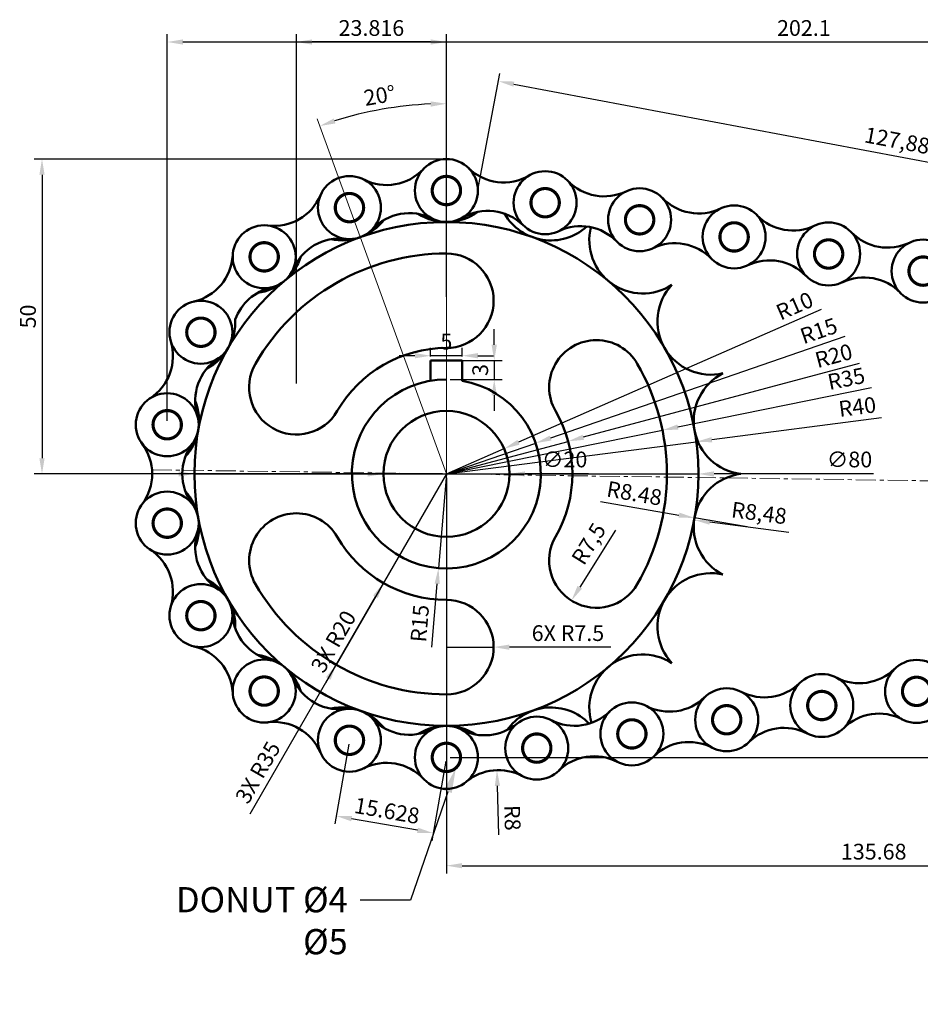
# Model space of a CAD drawing. Units: millimetres. Extents: x 3183 to 3437, y 1388 to 1545.
# Tile 1 of 2: x 3183 to 3326, y 1388 to 1545. Entities that reach past the tile are written whole.
import ezdxf
from ezdxf import colors
from ezdxf.entities.mleader import LeaderData, LeaderLine
from ezdxf.math import Vec2, Vec3

# ---------------------------------------------------------------- set-up
doc = ezdxf.new("R2010")
doc.units = ezdxf.units.MM
doc.linetypes.add('CENTER', pattern=[50.8, 31.75, -6.35, 6.35, -6.35])
for name, color, linetype, lineweight in [('M-CNTR', 1, 'CENTER', 18), ('M-CONS', 8, 'Continuous', 13), ('M-DIMS', 2, 'Continuous', 25), ('M-OUTL', 7, 'Continuous', 50)]:
    doc.layers.add(name, color=color, linetype=linetype, lineweight=lineweight)
doc.styles.get("Standard").update_dxf_attribs({"font": 'arial.ttf'})
doc.dimstyles.new('ISO-25', dxfattribs={"dimtxt": 2.5, "dimasz": 2.5, "dimexe": 1.25, "dimexo": 0.625, "dimtad": 1, "dimtxsty": 'Standard', "dimcen": 2.5, "dimadec": 0, "dimazin": 0, "dimtfac": 1, "dimtmove": 0, "dimatfit": 3, "dimfxl": 1, "dimarcsym": 0})

# ---------------------------------------------------------------- blocks, each defined once
blk = doc.blocks.new('*D6')
at = {"layer": 'Defpoints', "color": 0, "transparency": 16777216}
for p in [(3250.4, 1490.6), (3250.4, 1487.6), (3258, 1487.6)]:
    blk.add_point(p, dxfattribs=at)
at = {"layer": 'M-DIMS', "color": 0, "lineweight": -2, "transparency": 16777216}
for p, q in [((3258, 1493.1), (3258, 1495.6)), ((3251.03, 1490.6), (3259.25, 1490.6)), ((3258, 1490.6), (3258, 1487.6)), ((3251.03, 1487.6), (3259.25, 1487.6)), ((3258, 1485.1), (3258, 1482.6))]:
    blk.add_line(p, q, dxfattribs=at)
at = {"layer": 'M-DIMS', "color": 0, "transparency": 16777216}
for points in [[(3257.58, 1493.1), (3258.42, 1493.1), (3258, 1490.6)], [(3257.58, 1485.1), (3258.42, 1485.1), (3258, 1487.6)]]:
    blk.add_solid(points, dxfattribs=at)
at = {"layer": 'M-DIMS', "color": 0, "transparency": 16777216, "insert": (3256.1, 1489.1), "char_height": 2.5, "attachment_point": 5, "rotation": 90}
blk.add_mtext('3', dxfattribs=at)
blk = doc.blocks.new('*D7')
at = {"layer": 'Defpoints', "color": 0, "transparency": 16777216}
for p in [(3247.9, 1491.37), (3247.9, 1490.6), (3252.9, 1490.6)]:
    blk.add_point(p, dxfattribs=at)
at = {"layer": 'M-DIMS', "color": 0, "lineweight": -2, "transparency": 16777216}
for p, q in [((3247.9, 1491.22), (3247.9, 1492.62)), ((3252.9, 1491.22), (3252.9, 1492.62)), ((3245.4, 1491.37), (3242.9, 1491.37)), ((3252.9, 1491.37), (3247.9, 1491.37)), ((3255.4, 1491.37), (3257.9, 1491.37))]:
    blk.add_line(p, q, dxfattribs=at)
at = {"layer": 'M-DIMS', "color": 0, "transparency": 16777216}
for points in [[(3245.4, 1491.79), (3245.4, 1490.95), (3247.9, 1491.37)], [(3255.4, 1491.79), (3255.4, 1490.95), (3252.9, 1491.37)]]:
    blk.add_solid(points, dxfattribs=at)
at = {"layer": 'M-DIMS', "color": 0, "transparency": 16777216, "insert": (3250.4, 1493.27), "char_height": 2.5, "attachment_point": 5}
blk.add_mtext('5', dxfattribs=at)
blk = doc.blocks.new('*D1')
at = {"layer": 'Defpoints', "color": 0, "transparency": 16777216}
for p in [(3259.56, 1476.61), (3250.4, 1472.6)]:
    blk.add_point(p, dxfattribs=at)
at = {"layer": 'M-DIMS', "color": 0, "lineweight": -2, "transparency": 16777216}
for p, q in [((3309.88, 1498.69), (3261.85, 1477.62)), ((3250.4, 1472.6), (3259.56, 1476.61))]:
    blk.add_line(p, q, dxfattribs=at)
at = {"layer": 'M-DIMS', "color": 0, "transparency": 16777216}
blk.add_solid([(3261.68, 1478), (3262.02, 1477.24), (3259.56, 1476.61)], dxfattribs=at)
at = {"layer": 'M-DIMS', "color": 0, "transparency": 16777216, "insert": (3305.81, 1498.98), "char_height": 2.5, "attachment_point": 5, "rotation": 23.6896}
blk.add_mtext('R10', dxfattribs=at)
blk = doc.blocks.new('*D2')
at = {"layer": 'Defpoints', "color": 0, "transparency": 16777216}
for p in [(3264.59, 1477.49), (3250.4, 1472.6)]:
    blk.add_point(p, dxfattribs=at)
at = {"layer": 'M-DIMS', "color": 0, "lineweight": -2, "transparency": 16777216}
for p, q in [((3313.67, 1494.41), (3266.95, 1478.3)), ((3250.4, 1472.6), (3264.59, 1477.49))]:
    blk.add_line(p, q, dxfattribs=at)
at = {"layer": 'M-DIMS', "color": 0, "transparency": 16777216}
blk.add_solid([(3266.81, 1478.69), (3267.08, 1477.91), (3264.59, 1477.49)], dxfattribs=at)
at = {"layer": 'M-DIMS', "color": 0, "transparency": 16777216, "insert": (3309.62, 1495.02), "char_height": 2.5, "attachment_point": 5, "rotation": 19.0231}
blk.add_mtext('R15', dxfattribs=at)
blk = doc.blocks.new('*D3')
at = {"layer": 'Defpoints', "color": 0, "transparency": 16777216}
for p in [(3269.72, 1477.77), (3250.4, 1472.6)]:
    blk.add_point(p, dxfattribs=at)
at = {"layer": 'M-DIMS', "color": 0, "lineweight": -2, "transparency": 16777216}
for p, q in [((3315.94, 1490.15), (3272.14, 1478.42)), ((3250.4, 1472.6), (3269.72, 1477.77))]:
    blk.add_line(p, q, dxfattribs=at)
at = {"layer": 'M-DIMS', "color": 0, "transparency": 16777216}
blk.add_solid([(3272.03, 1478.82), (3272.25, 1478.01), (3269.72, 1477.77)], dxfattribs=at)
at = {"layer": 'M-DIMS', "color": 0, "transparency": 16777216, "insert": (3311.97, 1491.05), "char_height": 2.5, "attachment_point": 5, "rotation": 14.992}
blk.add_mtext('R20', dxfattribs=at)
blk = doc.blocks.new('*D4')
at = {"layer": 'Defpoints', "color": 0, "transparency": 16777216}
for p in [(3284.71, 1479.55), (3250.4, 1472.6)]:
    blk.add_point(p, dxfattribs=at)
at = {"layer": 'M-DIMS', "color": 0, "lineweight": -2, "transparency": 16777216}
for p, q in [((3317.88, 1486.27), (3287.16, 1480.04)), ((3250.4, 1472.6), (3284.71, 1479.55))]:
    blk.add_line(p, q, dxfattribs=at)
at = {"layer": 'M-DIMS', "color": 0, "transparency": 16777216}
blk.add_solid([(3287.08, 1480.45), (3287.24, 1479.63), (3284.71, 1479.55)], dxfattribs=at)
at = {"layer": 'M-DIMS', "color": 0, "transparency": 16777216, "insert": (3313.95, 1487.41), "char_height": 2.5, "attachment_point": 5, "rotation": 11.4531}
blk.add_mtext('R35', dxfattribs=at)
blk = doc.blocks.new('*D5')
at = {"layer": 'Defpoints', "color": 0, "transparency": 16777216}
for p in [(3290.08, 1477.71), (3250.4, 1472.6)]:
    blk.add_point(p, dxfattribs=at)
at = {"layer": 'M-DIMS', "color": 0, "lineweight": -2, "transparency": 16777216}
for p, q in [((3319.5, 1481.51), (3292.56, 1478.03)), ((3250.4, 1472.6), (3290.08, 1477.71))]:
    blk.add_line(p, q, dxfattribs=at)
at = {"layer": 'M-DIMS', "color": 0, "transparency": 16777216}
blk.add_solid([(3292.5, 1478.45), (3292.61, 1477.62), (3290.08, 1477.71)], dxfattribs=at)
at = {"layer": 'M-DIMS', "color": 0, "transparency": 16777216, "insert": (3315.68, 1482.94), "char_height": 2.5, "attachment_point": 5, "rotation": 7.3523}
blk.add_mtext('R40', dxfattribs=at)
blk = doc.blocks.new('*D10')
at = {"layer": 'Defpoints', "color": 0, "transparency": 16777216}
for p in [(3258.43, 1425.57), (3258.68, 1417.57)]:
    blk.add_point(p, dxfattribs=at)
at = {"layer": 'M-DIMS', "color": 0, "lineweight": -2, "transparency": 16777216}
blk.add_line((3258.75, 1415.28), (3258.5, 1423.07), dxfattribs=at)
at = {"layer": 'M-DIMS', "color": 0, "transparency": 16777216}
blk.add_solid([(3258.92, 1423.08), (3258.09, 1423.05), (3258.43, 1425.57)], dxfattribs=at)
at = {"layer": 'M-DIMS', "color": 0, "transparency": 16777216, "insert": (3260.57, 1417.99), "char_height": 2.5, "attachment_point": 5, "rotation": 271.825}
blk.add_mtext('R8', dxfattribs=at)
blk = doc.blocks.new('*D15')
at = {"layer": 'Defpoints', "color": 0, "transparency": 16777216}
for p in [(3255.4, 1517.6), (3384.35, 1511.3), (3381.08, 1493.94)]:
    blk.add_point(p, dxfattribs=at)
at = {"layer": 'M-DIMS', "color": 0, "lineweight": -2, "transparency": 16777216}
for p, q in [((3255.52, 1518.21), (3258.9, 1536.18)), ((3261.13, 1534.49), (3381.89, 1511.76)), ((3381.2, 1494.56), (3384.58, 1512.53))]:
    blk.add_line(p, q, dxfattribs=at)
at = {"layer": 'M-DIMS', "color": 0, "transparency": 16777216}
for points in [[(3261.2, 1534.9), (3261.05, 1534.08), (3258.67, 1534.95)], [(3381.97, 1512.17), (3381.81, 1511.35), (3384.35, 1511.3)]]:
    blk.add_solid(points, dxfattribs=at)
at = {"layer": 'M-DIMS', "color": 0, "transparency": 16777216, "insert": (3321.9, 1525.22), "char_height": 2.5, "attachment_point": 5, "rotation": 349.3415}
blk.add_mtext('127,88', dxfattribs=at)
blk = doc.blocks.new('*D16')
at = {"layer": 'Defpoints', "color": 0, "transparency": 16777216}
for p in [(3289.74, 1465.28), (3298.15, 1464.18)]:
    blk.add_point(p, dxfattribs=at)
at = {"layer": 'M-DIMS', "color": 0, "lineweight": -2, "transparency": 16777216}
blk.add_line((3304.75, 1463.31), (3292.22, 1464.95), dxfattribs=at)
at = {"layer": 'M-DIMS', "color": 0, "transparency": 16777216}
blk.add_solid([(3292.27, 1465.37), (3292.16, 1464.54), (3289.74, 1465.28)], dxfattribs=at)
at = {"layer": 'M-DIMS', "color": 0, "transparency": 16777216, "insert": (3300, 1466.08), "char_height": 2.5, "attachment_point": 5, "rotation": 352.5585}
blk.add_mtext('R8,48', dxfattribs=at)
blk = doc.blocks.new('*D17')
at = {"layer": 'Defpoints', "color": 0, "transparency": 16777216}
for p in [(3274.22, 1458.85), (3270.25, 1452.48)]:
    blk.add_point(p, dxfattribs=at)
at = {"layer": 'M-DIMS', "color": 0, "lineweight": -2, "transparency": 16777216}
blk.add_line((3277.24, 1463.69), (3271.58, 1454.6), dxfattribs=at)
at = {"layer": 'M-DIMS', "color": 0, "transparency": 16777216}
blk.add_solid([(3271.22, 1454.82), (3271.93, 1454.38), (3270.25, 1452.48)], dxfattribs=at)
at = {"layer": 'M-DIMS', "color": 0, "transparency": 16777216, "insert": (3273.27, 1461.33), "char_height": 2.5, "attachment_point": 5, "rotation": 58.0805}
blk.add_mtext('R7,5', dxfattribs=at)
blk = doc.blocks.new('*D18')
at = {"layer": 'Defpoints', "color": 0, "transparency": 16777216}
for p in [(3243.58, 1530.98), (3229.88, 1528.98), (3250.4, 1517.6), (3250.4, 1512.6), (3250.4, 1472.6)]:
    blk.add_point(p, dxfattribs=at)
at = {"layer": 'M-DIMS', "color": 0, "lineweight": -2, "transparency": 16777216}
blk.add_line((3250.4, 1518.22), (3250.4, 1532.63), dxfattribs=at)
blk.add_arc((3250.4, 1472.6), 58.79, 92.4368, 107.5632, dxfattribs=at)
at = {"layer": 'M-DIMS', "color": 0, "transparency": 16777216}
for points in [[(3247.9, 1531.75), (3247.91, 1530.91), (3250.4, 1531.38)], [(3232.8, 1528.25), (3232.53, 1529.04), (3230.3, 1527.84)]]:
    blk.add_solid(points, dxfattribs=at)
at = {"layer": 'M-DIMS', "color": 0, "transparency": 16777216, "insert": (3239.87, 1532.36), "char_height": 2.5, "attachment_point": 5, "rotation": 10}
blk.add_mtext('20°', dxfattribs=at)
blk = doc.blocks.new('*D19')
at = {"layer": 'Defpoints', "color": 0, "transparency": 16777216}
for p in [(3250.4, 1522.6), (3186.21, 1472.6), (3250.4, 1472.6)]:
    blk.add_point(p, dxfattribs=at)
at = {"layer": 'M-DIMS', "color": 0, "lineweight": -2, "transparency": 16777216}
for p, q in [((3249.78, 1522.6), (3184.96, 1522.6)), ((3186.21, 1520.1), (3186.21, 1475.1)), ((3249.78, 1472.6), (3184.96, 1472.6))]:
    blk.add_line(p, q, dxfattribs=at)
at = {"layer": 'M-DIMS', "color": 0, "transparency": 16777216}
for points in [[(3185.79, 1520.1), (3186.63, 1520.1), (3186.21, 1522.6)], [(3185.79, 1475.1), (3186.63, 1475.1), (3186.21, 1472.6)]]:
    blk.add_solid(points, dxfattribs=at)
at = {"layer": 'M-DIMS', "color": 0, "transparency": 16777216, "insert": (3184.31, 1497.6), "char_height": 2.5, "attachment_point": 5, "rotation": 90}
blk.add_mtext('50', dxfattribs=at)
blk = doc.blocks.new('CHAIN-ROLLER')
at = {"const_width": 0.5}
blk.add_lwpolyline([(3252.61, 1517.82, 1), (3248.13, 1517.37, 1)], format="xyb", close=True, dxfattribs=at)
blk.add_circle((3250.37, 1517.59), 5)
blk = doc.blocks.new('CHAIN-ROLLER-B')
at = {"const_width": 0.5}
blk.add_lwpolyline([(3262.52, 1429.27, -1), (3267, 1428.86, -1)], format="xyb", close=True, dxfattribs=at)
blk.add_circle((3264.76, 1429.06), 5)
blk = doc.blocks.new('*D22')
at = {"layer": 'Defpoints', "color": 0, "transparency": 16777216}
for p in [(3250.4, 1472.6), (3386.08, 1470.66), (3386.08, 1410.4)]:
    blk.add_point(p, dxfattribs=at)
at = {"layer": 'M-DIMS', "color": 0, "lineweight": -2, "transparency": 16777216}
for p, q in [((3250.4, 1471.97), (3250.4, 1409.15)), ((3386.08, 1470.04), (3386.08, 1409.15)), ((3252.9, 1410.4), (3383.58, 1410.4))]:
    blk.add_line(p, q, dxfattribs=at)
at = {"layer": 'M-DIMS', "color": 0, "transparency": 16777216}
for points in [[(3252.9, 1410.81), (3252.9, 1409.98), (3250.4, 1410.4)], [(3383.58, 1410.81), (3383.58, 1409.98), (3386.08, 1410.4)]]:
    blk.add_solid(points, dxfattribs=at)
at = {"layer": 'M-DIMS', "color": 0, "transparency": 16777216, "insert": (3318.24, 1412.3), "char_height": 2.5, "attachment_point": 5}
blk.add_mtext('135.68', dxfattribs=at)
blk = doc.blocks.new('*D23')
at = {"layer": 'Defpoints', "color": 0, "transparency": 16777216}
for p in [(3386.08, 1470.66), (3250.4, 1427.6), (3435.3, 1427.6)]:
    blk.add_point(p, dxfattribs=at)
at = {"layer": 'M-DIMS', "color": 0, "lineweight": -2, "transparency": 16777216}
for p, q in [((3386.7, 1470.66), (3436.55, 1470.66)), ((3435.3, 1468.16), (3435.3, 1430.1)), ((3251.03, 1427.6), (3436.55, 1427.6))]:
    blk.add_line(p, q, dxfattribs=at)
at = {"layer": 'M-DIMS', "color": 0, "transparency": 16777216}
for points in [[(3434.89, 1468.16), (3435.72, 1468.16), (3435.3, 1470.66)], [(3434.89, 1430.1), (3435.72, 1430.1), (3435.3, 1427.6)]]:
    blk.add_solid(points, dxfattribs=at)
at = {"layer": 'M-DIMS', "color": 0, "transparency": 16777216, "insert": (3433.4, 1449.13), "char_height": 2.5, "attachment_point": 5, "rotation": 90}
blk.add_mtext('43.07', dxfattribs=at)
blk = doc.blocks.new('*D24')
at = {"layer": 'Defpoints', "color": 0, "transparency": 16777216}
for p in [(3408.21, 1541.18), (3206.09, 1480.41), (3408.21, 1477.84)]:
    blk.add_point(p, dxfattribs=at)
at = {"layer": 'M-DIMS', "color": 0, "lineweight": -2, "transparency": 16777216}
for p, q in [((3206.09, 1481.04), (3206.09, 1542.43)), ((3408.21, 1478.47), (3408.21, 1542.43)), ((3208.59, 1541.18), (3405.71, 1541.18))]:
    blk.add_line(p, q, dxfattribs=at)
at = {"layer": 'M-DIMS', "color": 0, "transparency": 16777216}
for points in [[(3208.59, 1541.59), (3208.59, 1540.76), (3206.09, 1541.18)], [(3405.71, 1541.59), (3405.71, 1540.76), (3408.21, 1541.18)]]:
    blk.add_solid(points, dxfattribs=at)
at = {"layer": 'M-DIMS', "color": 0, "transparency": 16777216, "insert": (3307.15, 1543.08), "char_height": 2.5, "attachment_point": 5}
blk.add_mtext('202.1', dxfattribs=at)
blk = doc.blocks.new('*D25')
at = {"layer": 'Defpoints', "color": 0, "transparency": 16777216}
for p in [(3235.01, 1430.31), (3250.4, 1427.6), (3232.9, 1418.3)]:
    blk.add_point(p, dxfattribs=at)
at = {"layer": 'M-DIMS', "color": 0, "lineweight": -2, "transparency": 16777216}
for p, q in [((3234.91, 1429.69), (3232.68, 1417.06)), ((3250.3, 1426.98), (3248.07, 1414.35)), ((3245.82, 1416.02), (3235.36, 1417.86))]:
    blk.add_line(p, q, dxfattribs=at)
at = {"layer": 'M-DIMS', "color": 0, "transparency": 16777216}
for points in [[(3235.43, 1418.27), (3235.28, 1417.45), (3232.9, 1418.3)], [(3245.9, 1416.43), (3245.75, 1415.6), (3248.29, 1415.58)]]:
    blk.add_solid(points, dxfattribs=at)
at = {"layer": 'M-DIMS', "color": 0, "transparency": 16777216, "insert": (3240.92, 1418.81), "char_height": 2.5, "attachment_point": 5, "rotation": 350}
blk.add_mtext('15.628', dxfattribs=at)
blk = doc.blocks.new('*D27')
at = {"layer": 'Defpoints', "color": 0, "transparency": 16777216}
for p in [(3226.59, 1541.18), (3250.4, 1500.1), (3226.59, 1486.35)]:
    blk.add_point(p, dxfattribs=at)
at = {"layer": 'M-DIMS', "color": 0, "lineweight": -2, "transparency": 16777216}
for p, q in [((3226.59, 1486.97), (3226.59, 1542.43)), ((3250.4, 1500.72), (3250.4, 1542.43)), ((3247.9, 1541.18), (3229.09, 1541.18))]:
    blk.add_line(p, q, dxfattribs=at)
at = {"layer": 'M-DIMS', "color": 0, "transparency": 16777216}
for points in [[(3229.09, 1541.59), (3229.09, 1540.76), (3226.59, 1541.18)], [(3247.9, 1541.59), (3247.9, 1540.76), (3250.4, 1541.18)]]:
    blk.add_solid(points, dxfattribs=at)
at = {"layer": 'M-DIMS', "color": 0, "transparency": 16777216, "insert": (3238.5, 1543.08), "char_height": 2.5, "attachment_point": 5}
blk.add_mtext('23.816', dxfattribs=at)
blk = doc.blocks.new('*D28')
at = {"layer": 'Defpoints', "color": 0, "transparency": 16777216}
for p in [(3210.4, 1472.6), (3290.4, 1472.6)]:
    blk.add_point(p, dxfattribs=at)
at = {"layer": 'M-DIMS', "color": 0, "lineweight": -2, "transparency": 16777216}
for p, q in [((3207.9, 1472.6), (3205.4, 1472.6)), ((3210.4, 1472.6), (3290.4, 1472.6)), ((3318.18, 1472.6), (3292.9, 1472.6))]:
    blk.add_line(p, q, dxfattribs=at)
at = {"layer": 'M-DIMS', "color": 0, "transparency": 16777216}
for points in [[(3207.9, 1473.01), (3207.9, 1472.18), (3210.4, 1472.6)], [(3292.9, 1473.01), (3292.9, 1472.18), (3290.4, 1472.6)]]:
    blk.add_solid(points, dxfattribs=at)
at = {"layer": 'M-DIMS', "color": 0, "transparency": 16777216, "insert": (3314.4, 1474.57), "char_height": 2.5, "attachment_point": 5, "rotation": 0.0002}
blk.add_mtext('∅80', dxfattribs=at)
blk = doc.blocks.new('*D29')
at = {"layer": 'Defpoints', "color": 0, "transparency": 16777216}
for p in [(3250.4, 1472.6), (3232.9, 1442.28)]:
    blk.add_point(p, dxfattribs=at)
at = {"layer": 'M-DIMS', "color": 0, "lineweight": -2, "transparency": 16777216}
for p, q in [((3250.4, 1472.6), (3232.9, 1442.28)), ((3219.25, 1418.64), (3231.65, 1440.12))]:
    blk.add_line(p, q, dxfattribs=at)
at = {"layer": 'M-DIMS', "color": 0, "transparency": 16777216}
blk.add_solid([(3231.29, 1440.33), (3232.02, 1439.91), (3232.9, 1442.28)], dxfattribs=at)
at = {"layer": 'M-DIMS', "color": 0, "transparency": 16777216, "insert": (3220.76, 1425.05), "char_height": 2.5, "attachment_point": 5, "rotation": 60.0005}
blk.add_mtext('3X R35', dxfattribs=at)
blk = doc.blocks.new('*D30')
at = {"layer": 'Defpoints', "color": 0, "transparency": 16777216}
for p in [(3250.4, 1472.6), (3240.41, 1455.28)]:
    blk.add_point(p, dxfattribs=at)
at = {"layer": 'M-DIMS', "color": 0, "lineweight": -2, "transparency": 16777216}
for p, q in [((3250.4, 1472.6), (3240.41, 1455.28)), ((3231.26, 1439.43), (3239.16, 1453.11))]:
    blk.add_line(p, q, dxfattribs=at)
at = {"layer": 'M-DIMS', "color": 0, "transparency": 16777216}
blk.add_solid([(3238.79, 1453.32), (3239.52, 1452.9), (3240.41, 1455.28)], dxfattribs=at)
at = {"layer": 'M-DIMS', "color": 0, "transparency": 16777216, "insert": (3232.76, 1445.83), "char_height": 2.5, "attachment_point": 5, "rotation": 60.0014}
blk.add_mtext('3X R20', dxfattribs=at)
blk = doc.blocks.new('*D31')
at = {"layer": 'Defpoints', "color": 0, "transparency": 16777216}
for p in [(3250.4, 1445.1), (3257.9, 1445.1)]:
    blk.add_point(p, dxfattribs=at)
at = {"layer": 'M-DIMS', "color": 0, "lineweight": -2, "transparency": 16777216}
for p, q in [((3250.4, 1445.1), (3257.9, 1445.1)), ((3276.5, 1445.1), (3260.4, 1445.1))]:
    blk.add_line(p, q, dxfattribs=at)
at = {"layer": 'M-DIMS', "color": 0, "transparency": 16777216}
blk.add_solid([(3260.4, 1445.51), (3260.4, 1444.68), (3257.9, 1445.1)], dxfattribs=at)
at = {"layer": 'M-DIMS', "color": 0, "transparency": 16777216, "insert": (3269.7, 1447), "char_height": 2.5, "attachment_point": 5, "rotation": 0.0013}
blk.add_mtext('6X R7.5', dxfattribs=at)
blk = doc.blocks.new('*D32')
at = {"layer": 'Defpoints', "color": 0, "transparency": 16777216}
for p in [(3250.4, 1472.6), (3249.15, 1457.65)]:
    blk.add_point(p, dxfattribs=at)
at = {"layer": 'M-DIMS', "color": 0, "lineweight": -2, "transparency": 16777216}
for p, q in [((3250.4, 1472.6), (3249.15, 1457.65)), ((3248.09, 1445.07), (3248.94, 1455.16))]:
    blk.add_line(p, q, dxfattribs=at)
at = {"layer": 'M-DIMS', "color": 0, "transparency": 16777216}
blk.add_solid([(3248.53, 1455.19), (3249.36, 1455.12), (3249.15, 1457.65)], dxfattribs=at)
at = {"layer": 'M-DIMS', "color": 0, "transparency": 16777216, "insert": (3246.5, 1448.84), "char_height": 2.5, "attachment_point": 5, "rotation": 85.2023}
blk.add_mtext('R15', dxfattribs=at)
blk = doc.blocks.new('*D33')
at = {"layer": 'Defpoints', "color": 0, "transparency": 16777216}
for p in [(3240.4, 1472.6), (3260.4, 1472.6)]:
    blk.add_point(p, dxfattribs=at)
at = {"layer": 'M-DIMS', "color": 0, "lineweight": -2, "transparency": 16777216}
for p, q in [((3237.9, 1472.6), (3235.4, 1472.6)), ((3240.4, 1472.6), (3260.4, 1472.6)), ((3272.95, 1472.6), (3262.9, 1472.6))]:
    blk.add_line(p, q, dxfattribs=at)
at = {"layer": 'M-DIMS', "color": 0, "transparency": 16777216}
for points in [[(3237.9, 1473.01), (3237.9, 1472.18), (3240.4, 1472.6)], [(3262.9, 1473.01), (3262.9, 1472.18), (3260.4, 1472.6)]]:
    blk.add_solid(points, dxfattribs=at)
at = {"layer": 'M-DIMS', "color": 0, "transparency": 16777216, "insert": (3269.18, 1474.57), "char_height": 2.5, "attachment_point": 5, "rotation": 0.0009}
blk.add_mtext('∅20', dxfattribs=at)
blk = doc.blocks.new('*D34')
at = {"layer": 'Defpoints', "color": 0, "transparency": 16777216}
for p in [(3289.79, 1465.62), (3298.15, 1464.18)]:
    blk.add_point(p, dxfattribs=at)
at = {"layer": 'M-DIMS', "color": 0, "lineweight": -2, "transparency": 16777216}
for p, q in [((3274.87, 1468.2), (3287.33, 1466.05)), ((3298.15, 1464.18), (3289.79, 1465.62))]:
    blk.add_line(p, q, dxfattribs=at)
at = {"layer": 'M-DIMS', "color": 0, "transparency": 16777216}
blk.add_solid([(3287.4, 1466.46), (3287.26, 1465.64), (3289.79, 1465.62)], dxfattribs=at)
at = {"layer": 'M-DIMS', "color": 0, "transparency": 16777216, "insert": (3280.19, 1469.21), "char_height": 2.5, "attachment_point": 5, "rotation": 350.1886}
blk.add_mtext('R8.48', dxfattribs=at)

msp = doc.modelspace()

# ---------------------------------------------------------------- linework, layer by layer
at = {"layer": 'M-CNTR'}
for p, q in [((3250.4046, 1512.5958), (3250.4046, 1517.5958)), ((3250.4046, 1432.5958), (3250.4046, 1427.5958))]:
    msp.add_line(p, q, dxfattribs=at)
at = {"layer": 'M-CNTR', "ltscale": 0.1}
msp.add_line((3250.4046, 1422.5958), (3250.4046, 1512.5958), dxfattribs=at)
msp.add_lwpolyline([(3203.6712, 1473.2614), (3386.08, 1470.6636), (3423.1034, 1470.6522)], dxfattribs=at)
at = {"layer": 'M-CONS'}
for q in [(3229.8834, 1528.9774), (3250.4046, 1512.5958)]:
    msp.add_line((3250.4046, 1472.5958), q, dxfattribs=at)
at = {"layer": 'M-OUTL'}
for p, q in [((3250.4046, 1490.5958), (3247.9046, 1490.5958)), ((3247.9046, 1490.5958), (3247.9046, 1487.386)), ((3250.4046, 1490.5958), (3252.9046, 1490.5958)), ((3252.9046, 1490.5958), (3252.9046, 1487.386))]:
    msp.add_line(p, q, dxfattribs=at)
for radius in [40, 10]:
    msp.add_circle((3250.4046, 1472.5958), radius, dxfattribs=at)
for centre, radius, start, end in [((3259.5056, 1526.8787), 8, 225.566575, 300.379061), ((3240.9051, 1526.4704), 8, 243.052008, 316.947992), ((3250.4046, 1521.0758), 8.48, 196.906667, 197.029407), ((3233.8235, 1518.1521), 8.48, 2.970593, 3.093333), ((3275.4557, 1524.669), 8, 223.845854, 295.635223), ((3223.0518, 1519.9724), 8, 263.052008, 336.947992), ((3290.4557, 1521.954), 8, 223.845854, 295.635223), ((3244.5132, 1506.0074), 8, 63.052008, 136.947992), ((3250.4046, 1521.0758), 8.48, 238.000421, 306.092204), ((3256.979, 1506.3808), 8, 45.566575, 120.379061), ((3266.9857, 1518.1521), 8.48, 209.878473, 312.3163), ((3305.4557, 1519.239), 8, 223.845854, 295.635223), ((3233.8235, 1518.1521), 8.48, 216.906667, 217.029407), ((3219.2423, 1509.7337), 8.48, 22.970593, 23.093333), ((3233.8235, 1518.1521), 8.48, 258.000421, 321.999579), ((3271.7043, 1503.9432), 8, 43.845854, 115.635223), ((3281.567, 1509.7337), 8.48, 166.070857, 303.093333), ((3256.979, 1506.3808), 8, 28.632649, 28.639026), ((3320.4557, 1516.524), 8, 223.845854, 295.635223), ((3233.4411, 1501.9775), 8, 83.052008, 156.947992), ((3286.7043, 1501.2282), 8, 43.845854, 115.635223), ((3208.4976, 1507.76), 8, 283.052008, 356.947992), ((3250.4046, 1472.5958), 35, 90, 150), ((3219.2423, 1509.7337), 8.48, 278.000421, 341.999579), ((3250.4046, 1500.0958), 7.5, 270, 90), ((3301.7043, 1498.5132), 8, 43.845854, 115.635223), ((3219.2423, 1509.7337), 8.48, 236.906667, 237.029407), ((3208.4197, 1496.8358), 8.48, 42.970593, 43.093333), ((3292.3895, 1496.8358), 8.48, 136.906667, 283.093333), ((3316.7043, 1495.7982), 8, 43.845854, 115.635223), ((3224.415, 1494.4037), 8, 103.052008, 160.061909), ((3208.4197, 1496.8358), 8.48, 298.000421, 1.999579), ((3198.9981, 1491.3063), 8, 303.052008, 16.947992), ((3274.2203, 1486.3458), 7.5, 30, 210), ((3286.7043, 1501.2282), 8, 253.864276, 254.65671), ((3250.4046, 1472.5958), 20, 90, 150), ((3218.5237, 1484.1995), 8, 123.052008, 196.947992), ((3226.5889, 1486.3458), 7.5, 150, 330), ((3250.4046, 1472.5958), 35, 330, 30), ((3208.4197, 1496.8358), 8.48, 256.906667, 257.029407), ((3202.6611, 1481.0143), 8.48, 62.970593, 63.093333), ((3298.1481, 1481.0143), 8.48, 116.906667, 263.093333), ((3250.4046, 1472.5958), 15, 90, 80.405932), ((3202.6611, 1481.0143), 8.48, 318.000421, 21.999579), ((3250.4046, 1472.5958), 20, 330, 30), ((3195.6989, 1472.5958), 8, 323.052008, 36.947992), ((3216.4776, 1472.5958), 8, 143.052008, 216.947992), ((3202.6611, 1481.0143), 8.48, 276.906667, 277.029407), ((3202.6611, 1464.1774), 8.48, 82.970593, 83.093333), ((3298.1481, 1464.1774), 8.48, 96.906667, 243.093333), ((3202.6611, 1464.1774), 8.48, 338.000421, 41.999579), ((3226.5889, 1458.8458), 7.5, 30, 210), ((3218.5237, 1460.9921), 8, 163.052008, 236.947992), ((3250.4046, 1472.5958), 20, 210, 270), ((3274.2203, 1458.8458), 7.5, 150, 330), ((3198.9981, 1453.8854), 8, 343.052008, 56.947992), ((3202.6611, 1464.1774), 8.48, 296.906667, 297.029407), ((3208.4197, 1448.3558), 8.48, 102.970593, 103.093333), ((3208.4197, 1448.3558), 8.48, 358.000421, 61.999579), ((3292.3895, 1448.3558), 8.48, 76.906667, 223.093333), ((3250.4046, 1472.5958), 35, 210, 270), ((3250.4046, 1445.0958), 7.5, 270, 90), ((3224.415, 1450.788), 8, 183.052008, 256.947992), ((3285.8069, 1442.861), 8, 103.581598, 104.374031), ((3208.4976, 1437.4317), 8, 3.052008, 76.947992), ((3219.2423, 1435.458), 8.48, 18.000421, 81.999579), ((3281.567, 1435.458), 8.48, 56.906667, 196.306861), ((3208.4197, 1448.3558), 8.48, 316.906667, 317.029407), ((3219.2423, 1435.458), 8.48, 122.970593, 123.093333), ((3315.9597, 1447.3662), 8, 242.603084, 314.392454), ((3233.4411, 1443.2142), 8, 195.167319, 276.947992), ((3300.8833, 1445.1136), 8, 242.603084, 314.392454), ((3285.8069, 1442.861), 8, 242.603084, 314.392454), ((3233.8235, 1427.0395), 8.48, 38.000421, 101.999579), ((3266.9857, 1427.0395), 8.48, 44.237712, 144.645339), ((3244.5132, 1439.1843), 8, 223.052008, 296.947992), ((3255.9372, 1438.6248), 8, 329.599281, 329.605658), ((3270.7305, 1440.6085), 8, 242.603084, 314.392454), ((3319.0721, 1426.5349), 8, 62.603084, 134.392454), ((3223.0518, 1425.2193), 8, 23.052008, 96.947992), ((3219.2423, 1435.458), 8.48, 336.906667, 337.029407), ((3233.8235, 1427.0395), 8.48, 142.970593, 143.093333), ((3250.4046, 1424.1158), 8.48, 56.951486, 121.999579), ((3256.4732, 1439.0924), 8, 242.172129, 309.53614), ((3303.9957, 1424.2824), 8, 62.603084, 134.392454), ((3288.9193, 1422.0298), 8, 62.603084, 134.392454), ((3273.843, 1419.7772), 8, 62.603084, 134.392454), ((3240.9051, 1418.7212), 8, 43.052008, 116.947992), ((3233.8235, 1427.0395), 8.48, 356.906667, 357.029407), ((3250.4046, 1424.1158), 8.48, 162.970593, 163.093333), ((3258.68, 1417.5699), 8, 62.172129, 129.53614)]:
    msp.add_arc(centre, radius, start, end, dxfattribs=at)

# ---------------------------------------------------------------- block references
for name, p, rotation in [('CHAIN-ROLLER', (6635.8449, 2703.6791), 174.2800065540521), ('CHAIN-ROLLER', (6651.5203, 2701.7468), 174.2800065539874), ('CHAIN-ROLLER', (6620.454, 2700.9652), 174.2800065540586), ('CHAIN-ROLLER', (6666.5203, 2699.0318), 174.2800065540113), ('CHAIN-ROLLER', (6681.5203, 2696.3168), 174.2800065540223), ('CHAIN-ROLLER', (6606.9194, 2693.1511), 174.2800065540527), ('CHAIN-ROLLER', (6696.5203, 2693.6018), 174.2800065540229), ('CHAIN-ROLLER', (6711.5203, 2690.8868), 174.2800065540113), ('CHAIN-ROLLER', (6596.8737, 2681.1791), 174.2800065540625), ('CHAIN-ROLLER', (6591.5285, 2666.4932), 174.2800065540643), ('CHAIN-ROLLER', (6591.5285, 2650.8649), 174.2800065541736), ('CHAIN-ROLLER', (6596.8737, 2636.1791), 174.2800065541353), ('CHAIN-ROLLER', (6606.9194, 2624.2071), 174.280006554112), ('CHAIN-ROLLER-B', (151.0164, -182.5314), 3.407903634794214), ('CHAIN-ROLLER-B', (120.8636, -187.0365), 3.407903634803631), ('CHAIN-ROLLER', (6620.454, 2616.3929), 174.2800065540305), ('CHAIN-ROLLER-B', (90.7109, -191.5417), 3.407903634793037), ('CHAIN-ROLLER', (6635.8449, 2613.6791), 174.2800065540637)]:
    msp.add_blockref(name, p, dxfattribs=dict(at, rotation=rotation))
at = {"layer": 'M-OUTL', "extrusion": (0, 0, -1), "zscale": -1, "rotation": 180.1085086200339}
for p in [(-47.9534, 2871.0723), (-17.8006, 2866.5671)]:
    msp.add_blockref('CHAIN-ROLLER-B', p, dxfattribs=at)

# ---------------------------------------------------------------- dimensions: what is measured, and where the dimension line sits
at = {"layer": 'M-DIMS'}
for base, p1, p2, override, picture, middle in [((3408.2054, 1541.1774), (3206.0883, 1480.41), (3408.2054, 1477.841), {"dimdec": 1, "dimlfac": 1, "dimrnd": 0, "dimzin": 0, "dimdsep": 46, "dimlunit": 2}, '*D24', (3307.1468, 1543.0788)), ((3226.5889, 1541.1774), (3250.4046, 1500.0958), (3226.5889, 1486.3458), {"dimdec": 3, "dimlfac": 1, "dimrnd": 0, "dimzin": 0, "dimdsep": 46, "dimlunit": 2}, '*D27', (3238.4968, 1543.0797)), ((3247.9046, 1491.3704), (3252.9046, 1490.5958), (3247.9046, 1490.5958), {"dimclrd": 0, "dimclre": 0, "dimclrt": 0}, '*D7', (3250.4046, 1493.2667)), ((3386.08, 1410.3958), (3250.4046, 1472.5958), (3386.08, 1470.6636), {"dimdec": 2, "dimlfac": 1, "dimrnd": 0, "dimzin": 0, "dimdsep": 46, "dimlunit": 2}, '*D22', (3318.2423, 1412.2981))]:
    dim = msp.add_linear_dim(base=base, p1=p1, p2=p2, dimstyle='ISO-25', override=override, dxfattribs=at)
    dim.commit()
    dim.dimension.update_dxf_attribs({"geometry": picture, "text_midpoint": middle})
dim = msp.add_aligned_dim(p1=(3255.4046, 1517.5958), p2=(3381.08, 1493.9436), distance=17.6603, dimstyle='ISO-25', override={"dimclrd": 0, "dimclre": 0, "dimclrt": 0}, dxfattribs=at)
dim.commit()
dim.dimension.update_dxf_attribs({"geometry": '*D15', "text_midpoint": (3321.9021, 1525.216)})
dim = msp.add_angular_dim_2l(base=(3243.5799, 1530.9846), line1=((3250.4046, 1472.5958), (3229.8834, 1528.9774)), line2=((3250.4046, 1512.5958), (3250.4046, 1517.5958)), dimstyle='ISO-25', override={"dimclrd": 0, "dimclre": 0, "dimclrt": 0}, dxfattribs=at)
dim.commit()
dim.dimension.update_dxf_attribs({"geometry": '*D18', "text_midpoint": (3239.8663, 1532.3615)})
for base, p1, p2, angle, override, picture, middle in [((3186.2111, 1472.5958), (3250.4046, 1522.5958), (3250.4046, 1472.5958), 90, {"dimclrd": 0, "dimclre": 0, "dimclrt": 0}, '*D19', (3184.3097, 1497.5958)), ((3258.0012, 1487.5958), (3250.4046, 1490.5958), (3250.4046, 1487.5958), 90, {"dimclrd": 0, "dimclre": 0, "dimclrt": 0}, '*D6', (3256.0989, 1489.0958)), ((3435.3034, 1427.5958), (3386.08, 1470.6636), (3250.4046, 1427.5958), 90, {"dimdec": 2, "dimlfac": 1, "dimrnd": 0, "dimzin": 0, "dimdsep": 46, "dimlunit": 2}, '*D23', (3433.4011, 1449.1297)), ((3232.8952, 1418.295), (3250.4046, 1427.5958), (3235.0137, 1430.3097), 170, {"dimdec": 3, "dimlfac": 1, "dimrnd": 0, "dimzin": 0, "dimdsep": 46, "dimlunit": 2}, '*D25', (3240.9208, 1418.8106))]:
    dim = msp.add_linear_dim(base=base, p1=p1, p2=p2, angle=angle, dimstyle='ISO-25', override=override, dxfattribs=at)
    dim.commit()
    dim.dimension.update_dxf_attribs({"geometry": picture, "text_midpoint": middle})
for center, mpoint, override, picture, middle in [((3250.4046, 1472.5958), (3259.562, 1476.6137), {"dimclrd": 0, "dimclre": 0, "dimclrt": 0}, '*D1', (3306.5726, 1497.2397)), ((3250.4046, 1472.5958), (3264.5854, 1477.4851), {"dimclrd": 0, "dimclre": 0, "dimclrt": 0}, '*D2', (3310.2426, 1493.2267)), ((3250.4046, 1472.5958), (3269.7239, 1477.7695), {"dimclrd": 0, "dimclre": 0, "dimclrt": 0}, '*D3', (3312.4584, 1489.2138)), ((3250.4046, 1472.5958), (3284.7077, 1479.5456), {"dimclrd": 0, "dimclre": 0, "dimclrt": 0}, '*D4', (3314.3281, 1485.5467)), ((3250.4046, 1472.5958), (3290.0757, 1477.7146), {"dimclrd": 0, "dimclre": 0, "dimclrt": 0}, '*D5', (3315.9207, 1481.0494)), ((3250.4046, 1472.5958), (3249.15, 1457.6484), {"dimdec": 0, "dimlfac": 1, "dimrnd": 0, "dimzin": 0, "dimdsep": 46, "dimlunit": 2}, '*D32', (3248.3973, 1448.6799)), ((3298.1481, 1464.1774), (3289.7395, 1465.2756), {"dimclrd": 0, "dimclre": 0, "dimclrt": 0}, '*D16', (3299.7255, 1463.9713)), ((3274.2203, 1458.8458), (3270.2549, 1452.4799), {"dimclrd": 0, "dimclre": 0, "dimclrt": 0}, '*D17', (3275.0697, 1460.2093)), ((3258.68, 1417.5699), (3258.4252, 1425.5659), {"dimclrd": 0, "dimclre": 0, "dimclrt": 0}, '*D10', (3258.6686, 1417.9265))]:
    dim = msp.add_radius_dim(center=center, mpoint=mpoint, dimstyle='ISO-25', override=override, dxfattribs=at)
    dim.commit()
    dim.dimension.update_dxf_attribs({"geometry": picture, "text_midpoint": middle, "dimtype": 164})
dim = msp.add_diameter_dim_2p(p1=(3210.4046, 1472.5957), p2=(3290.4046, 1472.596), dimstyle='ISO-25', override={"dimdec": 0, "dimlfac": 1, "dimrnd": 0, "dimzin": 0, "dimdsep": 46, "dimlunit": 2}, dxfattribs=at)
dim.commit()
dim.dimension.update_dxf_attribs({"geometry": '*D28', "text_midpoint": (3314.4046, 1472.5961), "dimtype": 163})
dim = msp.add_diameter_dim_2p(p1=(3240.4046, 1472.5957), p2=(3260.4046, 1472.596), dimstyle='ISO-25', override={"dimdec": 0, "dimlfac": 1, "dimrnd": 0, "dimzin": 0, "dimdsep": 46, "dimlunit": 2}, dxfattribs=at)
dim.commit()
dim.dimension.update_dxf_attribs({"geometry": '*D33', "text_midpoint": (3269.1759, 1472.5961)})
for mpoint, picture, middle in [((3232.9049, 1442.2848), '*D29', (3222.405, 1424.0982)), ((3240.405, 1455.2751), '*D30', (3234.4053, 1444.8826))]:
    dim = msp.add_radius_dim(center=(3250.4046, 1472.5958), mpoint=mpoint, text='3X <>', dimstyle='ISO-25', override={"dimdec": 0, "dimlfac": 1, "dimrnd": 0, "dimzin": 0, "dimdsep": 46, "dimlunit": 2}, dxfattribs=at)
    dim.commit()
    dim.dimension.update_dxf_attribs({"geometry": picture, "text_midpoint": middle, "dimtype": 164})
dim = msp.add_radius_dim(center=(3298.1481, 1464.1774), mpoint=(3289.7921, 1465.6224), dimstyle='ISO-25', override={"dimdec": 2, "dimlfac": 1, "dimrnd": 0, "dimzin": 0, "dimdsep": 46, "dimlunit": 2}, dxfattribs=at)
dim.commit()
dim.dimension.update_dxf_attribs({"geometry": '*D34', "text_midpoint": (3280.1927, 1469.2122)})
dim = msp.add_radius_dim(center=(3250.4046, 1445.0958), mpoint=(3257.9046, 1445.096), text='6X <>', dimstyle='ISO-25', override={"dimdec": 1, "dimlfac": 1, "dimrnd": 0, "dimzin": 0, "dimdsep": 46, "dimlunit": 2}, dxfattribs=at)
dim.commit()
dim.dimension.update_dxf_attribs({"geometry": '*D31', "text_midpoint": (3269.7037, 1446.9977)})

# ---------------------------------------------------------------- leaders
ml = msp.add_multileader_mtext('Standard', dxfattribs=at)
ml.set_content('DONUT %%C4\\P%%C5', color=256)
ml.set_leader_properties()
ml.build(insert=Vec2(0, 0))
ctx = ml.context
ctx.base_point, ctx.plane_origin = Vec3(3204.5604, 1404.9173), Vec3(3251.9196, 1425.9323)
ctx.text_align_type = 2
notes = []
notes.append((ctx, [(0, (1, 1, 0), (3244.7323, 1404.9173), (-1, 0), 8, [(0, [(3251.9196, 1425.9323)], 0, [])])]))
ctx.mtext.insert, ctx.mtext.alignment, ctx.mtext.flow_direction = Vec3(3234.7323, 1406.9978), 3, 5
for ctx, leaders in notes:
    for number, flags, end, landing, length, lines in leaders:
        leader = LeaderData()
        leader.index, (leader.has_last_leader_line, leader.has_dogleg_vector, leader.attachment_direction) = number, flags
        leader.last_leader_point, leader.dogleg_vector, leader.dogleg_length = Vec3(end), Vec3(landing), length
        for number, points, colour, breaks in lines:
            line = LeaderLine()
            line.index, line.vertices, line.color, line.breaks = number, Vec3.list(points), colors.encode_raw_color(colour), breaks
            leader.lines.append(line)
        ctx.leaders.append(leader)

doc.saveas('drawing.dxf')
